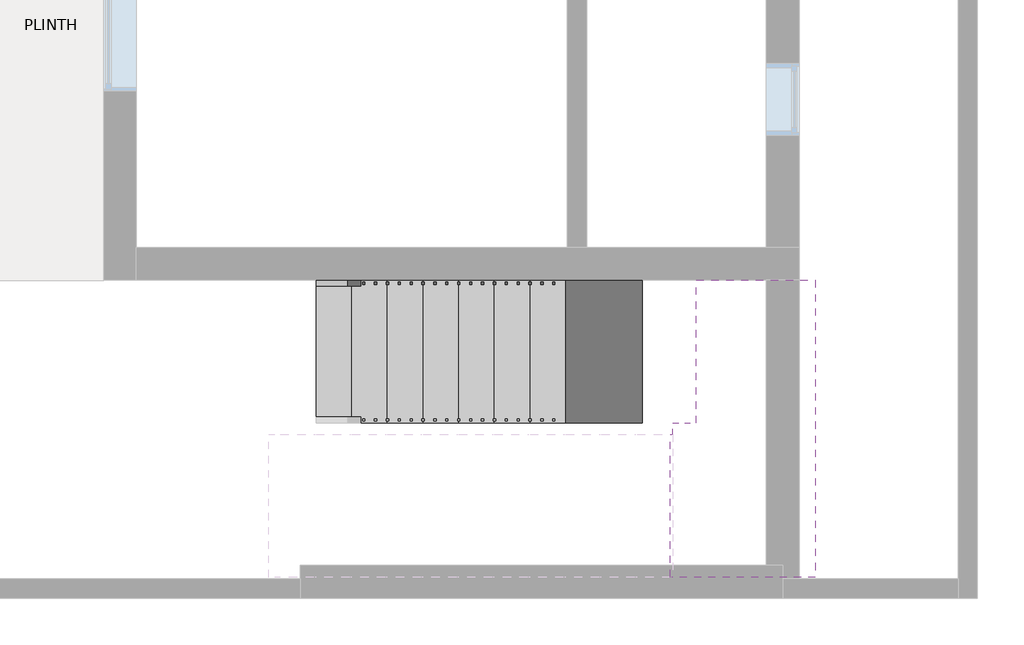
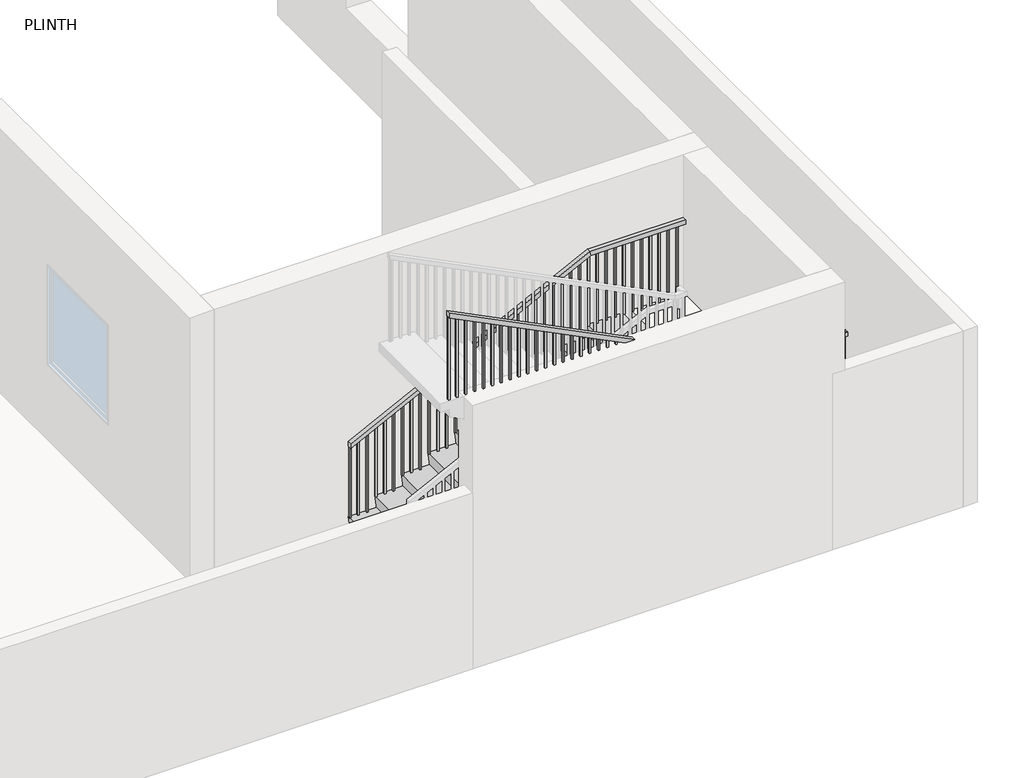
# One storey, part 3 of 3: 1 railing, 1 slab, 1 stair flight.
"""IFC4 building model written with IfcOpenShell, lengths in millimetres."""

from ifc_helpers import new_model, si_unit, frame, origin, place, context, project, spatial, polyline, outline, extrude, faceted_brep, element, save

model = new_model("IFC4")

# Units and contexts
model_context = context("Model", 3, world=origin())
ifc_project = project(units=[si_unit("LENGTHUNIT", "METRE", prefix="MILLI")], contexts=[model_context])

# Site, building, storey
site = spatial("IfcSite", under=ifc_project)
building = spatial("IfcBuilding", under=site)
storey = spatial("IfcBuildingStorey", under=building, Name="PLINTH", Elevation=0.0)

# Railing
placement = place(None, origin())
element("IfcRailing", 1, ObjectType="Handrail - Rectangular", at=placement, inside=storey, context=model_context, shape_type="SolidModel", body=[
    faceted_brep([(-13267.32252, -2786.4806156, 1066.8), (-13267.32252, -2786.4806156, 1010.0038734), (-13267.32252, -2837.2806156, 1010.0038734), (-13267.32252, -2837.2806156, 1066.8), (-10524.12252, -2786.4806156, 2438.4), (-10512.1302667, -2786.4806156, 2387.6), (-10512.1302667, -2837.2806156, 2387.6), (-10524.12252, -2837.2806156, 2438.4), (-9000.12252, -2786.4806156, 2438.4), (-9000.12252, -2786.4806156, 2387.6), (-9050.92252, -2837.2806156, 2387.6), (-9050.92252, -2837.2806156, 2438.4), (-9000.12252, -5326.4806156, 2438.4), (-9000.12252, -5326.4806156, 2387.6), (-9050.92252, -5275.6806156, 2387.6), (-9050.92252, -5275.6806156, 2438.4), (-9914.52252, -5326.4806156, 2438.4), (-9926.5147732, -5326.4806156, 2387.6), (-9926.5147732, -5275.6806156, 2387.6), (-9914.52252, -5275.6806156, 2438.4), (-13572.12252, -5326.4806156, 4267.2), (-13572.12252, -5275.6806156, 4267.2), (-13572.12252, -5275.6806156, 4210.4038734), (-13572.12252, -5326.4806156, 4210.4038734)], [[[0, 1, 2, 3]], [[1, 0, 4, 5]], [[2, 1, 5, 6]], [[3, 2, 6, 7]], [[0, 3, 7, 4]], [[5, 4, 8, 9]], [[6, 5, 9, 10]], [[7, 6, 10, 11]], [[4, 7, 11, 8]], [[9, 8, 12, 13]], [[10, 9, 13, 14]], [[11, 10, 14, 15]], [[8, 11, 15, 12]], [[13, 12, 16, 17]], [[14, 13, 17, 18]], [[15, 14, 18, 19]], [[12, 15, 19, 16]], [[20, 21, 22, 23]], [[17, 16, 20, 23]], [[18, 17, 23, 22]], [[19, 18, 22, 21]], [[16, 19, 21, 20]]]),
    extrude(outline(polyline([(4164.3663734, -13480.04752), (3200.4, -13480.04752), (3200.4, -13460.99752), (4154.8413734, -13460.99752), (4164.3663734, -13480.04752)])), frame((0.0, -5310.6056156, 0.0), z_axis=(0.0, 1.0, 0.0), x_axis=(0.0, 0.0, 1.0)), (0.0, 0.0, 1.0), 19.05),
    extrude(outline(polyline([(4113.5663734, -13378.44752), (3200.4, -13378.44752), (3200.4, -13359.39752), (4104.0413734, -13359.39752), (4113.5663734, -13378.44752)])), frame((0.0, -5310.6056156, 0.0), z_axis=(0.0, 1.0, 0.0), x_axis=(0.0, 0.0, 1.0)), (0.0, 0.0, 1.0), 19.05),
    extrude(outline(polyline([(4062.7663734, -13276.84752), (3200.4, -13276.84752), (3200.4, -13257.79752), (4053.2413734, -13257.79752), (4062.7663734, -13276.84752)])), frame((0.0, -5310.6056156, 0.0), z_axis=(0.0, 1.0, 0.0), x_axis=(0.0, 0.0, 1.0)), (0.0, 0.0, 1.0), 19.05),
    extrude(outline(polyline([(4011.9663734, -13175.24752), (3048.0, -13175.24752), (3048.0, -13156.19752), (4002.4413734, -13156.19752), (4011.9663734, -13175.24752)])), frame((0.0, -5310.6056156, 0.0), z_axis=(0.0, 1.0, 0.0), x_axis=(0.0, 0.0, 1.0)), (0.0, 0.0, 1.0), 19.05),
    extrude(outline(polyline([(3961.1663734, -13073.64752), (3048.0, -13073.64752), (3048.0, -13054.59752), (3951.6413734, -13054.59752), (3961.1663734, -13073.64752)])), frame((0.0, -5310.6056156, 0.0), z_axis=(0.0, 1.0, 0.0), x_axis=(0.0, 0.0, 1.0)), (0.0, 0.0, 1.0), 19.05),
    extrude(outline(polyline([(3910.3663734, -12972.04752), (3048.0, -12972.04752), (3048.0, -12952.99752), (3900.8413734, -12952.99752), (3910.3663734, -12972.04752)])), frame((0.0, -5310.6056156, 0.0), z_axis=(0.0, 1.0, 0.0), x_axis=(0.0, 0.0, 1.0)), (0.0, 0.0, 1.0), 19.05),
    extrude(outline(polyline([(3859.5663734, -12870.44752), (2895.6, -12870.44752), (2895.6, -12851.39752), (3850.0413734, -12851.39752), (3859.5663734, -12870.44752)])), frame((0.0, -5310.6056156, 0.0), z_axis=(0.0, 1.0, 0.0), x_axis=(0.0, 0.0, 1.0)), (0.0, 0.0, 1.0), 19.05),
    extrude(outline(polyline([(3808.7663734, -12768.84752), (2895.6, -12768.84752), (2895.6, -12749.79752), (3799.2413734, -12749.79752), (3808.7663734, -12768.84752)])), frame((0.0, -5310.6056156, 0.0), z_axis=(0.0, 1.0, 0.0), x_axis=(0.0, 0.0, 1.0)), (0.0, 0.0, 1.0), 19.05),
    extrude(outline(polyline([(3757.9663734, -12667.24752), (2895.6, -12667.24752), (2895.6, -12648.19752), (3748.4413734, -12648.19752), (3757.9663734, -12667.24752)])), frame((0.0, -5310.6056156, 0.0), z_axis=(0.0, 1.0, 0.0), x_axis=(0.0, 0.0, 1.0)), (0.0, 0.0, 1.0), 19.05),
    extrude(outline(polyline([(3707.1663734, -12565.64752), (2743.2, -12565.64752), (2743.2, -12546.59752), (3697.6413734, -12546.59752), (3707.1663734, -12565.64752)])), frame((0.0, -5310.6056156, 0.0), z_axis=(0.0, 1.0, 0.0), x_axis=(0.0, 0.0, 1.0)), (0.0, 0.0, 1.0), 19.05),
    extrude(outline(polyline([(3656.3663734, -12464.04752), (2743.2, -12464.04752), (2743.2, -12444.99752), (3646.8413734, -12444.99752), (3656.3663734, -12464.04752)])), frame((0.0, -5310.6056156, 0.0), z_axis=(0.0, 1.0, 0.0), x_axis=(0.0, 0.0, 1.0)), (0.0, 0.0, 1.0), 19.05),
    extrude(outline(polyline([(3605.5663734, -12362.44752), (2743.2, -12362.44752), (2743.2, -12343.39752), (3596.0413734, -12343.39752), (3605.5663734, -12362.44752)])), frame((0.0, -5310.6056156, 0.0), z_axis=(0.0, 1.0, 0.0), x_axis=(0.0, 0.0, 1.0)), (0.0, 0.0, 1.0), 19.05),
    extrude(outline(polyline([(3554.7663734, -12260.84752), (2590.8, -12260.84752), (2590.8, -12241.79752), (3545.2413734, -12241.79752), (3554.7663734, -12260.84752)])), frame((0.0, -5310.6056156, 0.0), z_axis=(0.0, 1.0, 0.0), x_axis=(0.0, 0.0, 1.0)), (0.0, 0.0, 1.0), 19.05),
    extrude(outline(polyline([(3503.9663734, -12159.24752), (2590.8, -12159.24752), (2590.8, -12140.19752), (3494.4413734, -12140.19752), (3503.9663734, -12159.24752)])), frame((0.0, -5310.6056156, 0.0), z_axis=(0.0, 1.0, 0.0), x_axis=(0.0, 0.0, 1.0)), (0.0, 0.0, 1.0), 19.05),
    extrude(outline(polyline([(3453.1663734, -12057.64752), (2590.8, -12057.64752), (2590.8, -12038.59752), (3443.6413734, -12038.59752), (3453.1663734, -12057.64752)])), frame((0.0, -5310.6056156, 0.0), z_axis=(0.0, 1.0, 0.0), x_axis=(0.0, 0.0, 1.0)), (0.0, 0.0, 1.0), 19.05),
    extrude(outline(polyline([(3402.3663734, -11956.04752), (2438.4, -11956.04752), (2438.4, -11936.99752), (3392.8413734, -11936.99752), (3402.3663734, -11956.04752)])), frame((0.0, -5310.6056156, 0.0), z_axis=(0.0, 1.0, 0.0), x_axis=(0.0, 0.0, 1.0)), (0.0, 0.0, 1.0), 19.05),
    extrude(outline(polyline([(3351.5663734, -11854.44752), (2438.4, -11854.44752), (2438.4, -11835.39752), (3342.0413734, -11835.39752), (3351.5663734, -11854.44752)])), frame((0.0, -5310.6056156, 0.0), z_axis=(0.0, 1.0, 0.0), x_axis=(0.0, 0.0, 1.0)), (0.0, 0.0, 1.0), 19.05),
    extrude(outline(polyline([(3300.7663734, -11752.84752), (2438.4, -11752.84752), (2438.4, -11733.79752), (3291.2413734, -11733.79752), (3300.7663734, -11752.84752)])), frame((0.0, -5310.6056156, 0.0), z_axis=(0.0, 1.0, 0.0), x_axis=(0.0, 0.0, 1.0)), (0.0, 0.0, 1.0), 19.05),
    extrude(outline(polyline([(3249.9663734, -11651.24752), (2286.0, -11651.24752), (2286.0, -11632.19752), (3240.4413734, -11632.19752), (3249.9663734, -11651.24752)])), frame((0.0, -5310.6056156, 0.0), z_axis=(0.0, 1.0, 0.0), x_axis=(0.0, 0.0, 1.0)), (0.0, 0.0, 1.0), 19.05),
    extrude(outline(polyline([(3199.1663734, -11549.64752), (2286.0, -11549.64752), (2286.0, -11530.59752), (3189.6413734, -11530.59752), (3199.1663734, -11549.64752)])), frame((0.0, -5310.6056156, 0.0), z_axis=(0.0, 1.0, 0.0), x_axis=(0.0, 0.0, 1.0)), (0.0, 0.0, 1.0), 19.05),
    extrude(outline(polyline([(3148.3663734, -11448.04752), (2286.0, -11448.04752), (2286.0, -11428.99752), (3138.8413734, -11428.99752), (3148.3663734, -11448.04752)])), frame((0.0, -5310.6056156, 0.0), z_axis=(0.0, 1.0, 0.0), x_axis=(0.0, 0.0, 1.0)), (0.0, 0.0, 1.0), 19.05),
    extrude(outline(polyline([(3097.5663734, -11346.44752), (2133.6, -11346.44752), (2133.6, -11327.39752), (3088.0413734, -11327.39752), (3097.5663734, -11346.44752)])), frame((0.0, -5310.6056156, 0.0), z_axis=(0.0, 1.0, 0.0), x_axis=(0.0, 0.0, 1.0)), (0.0, 0.0, 1.0), 19.05),
    extrude(outline(polyline([(3046.7663734, -11244.84752), (2133.6, -11244.84752), (2133.6, -11225.79752), (3037.2413734, -11225.79752), (3046.7663734, -11244.84752)])), frame((0.0, -5310.6056156, 0.0), z_axis=(0.0, 1.0, 0.0), x_axis=(0.0, 0.0, 1.0)), (0.0, 0.0, 1.0), 19.05),
    extrude(outline(polyline([(2995.9663734, -11143.24752), (2133.6, -11143.24752), (2133.6, -11124.19752), (2986.4413734, -11124.19752), (2995.9663734, -11143.24752)])), frame((0.0, -5310.6056156, 0.0), z_axis=(0.0, 1.0, 0.0), x_axis=(0.0, 0.0, 1.0)), (0.0, 0.0, 1.0), 19.05),
    extrude(outline(polyline([(2945.1663734, -11041.64752), (1981.2, -11041.64752), (1981.2, -11022.59752), (2935.6413734, -11022.59752), (2945.1663734, -11041.64752)])), frame((0.0, -5310.6056156, 0.0), z_axis=(0.0, 1.0, 0.0), x_axis=(0.0, 0.0, 1.0)), (0.0, 0.0, 1.0), 19.05),
    extrude(outline(polyline([(2894.3663734, -10940.04752), (1981.2, -10940.04752), (1981.2, -10920.99752), (2884.8413734, -10920.99752), (2894.3663734, -10940.04752)])), frame((0.0, -5310.6056156, 0.0), z_axis=(0.0, 1.0, 0.0), x_axis=(0.0, 0.0, 1.0)), (0.0, 0.0, 1.0), 19.05),
    extrude(outline(polyline([(2843.5663734, -10838.44752), (1981.2, -10838.44752), (1981.2, -10819.39752), (2834.0413734, -10819.39752), (2843.5663734, -10838.44752)])), frame((0.0, -5310.6056156, 0.0), z_axis=(0.0, 1.0, 0.0), x_axis=(0.0, 0.0, 1.0)), (0.0, 0.0, 1.0), 19.05),
    extrude(outline(polyline([(2792.7663734, -10736.84752), (1828.8, -10736.84752), (1828.8, -10717.79752), (2783.2413734, -10717.79752), (2792.7663734, -10736.84752)])), frame((0.0, -5310.6056156, 0.0), z_axis=(0.0, 1.0, 0.0), x_axis=(0.0, 0.0, 1.0)), (0.0, 0.0, 1.0), 19.05),
    extrude(outline(polyline([(2741.9663734, -10635.24752), (1828.8, -10635.24752), (1828.8, -10616.19752), (2732.4413734, -10616.19752), (2741.9663734, -10635.24752)])), frame((0.0, -5310.6056156, 0.0), z_axis=(0.0, 1.0, 0.0), x_axis=(0.0, 0.0, 1.0)), (0.0, 0.0, 1.0), 19.05),
    extrude(outline(polyline([(2691.1663734, -10533.64752), (1828.8, -10533.64752), (1828.8, -10514.59752), (2681.6413734, -10514.59752), (2691.1663734, -10533.64752)])), frame((0.0, -5310.6056156, 0.0), z_axis=(0.0, 1.0, 0.0), x_axis=(0.0, 0.0, 1.0)), (0.0, 0.0, 1.0), 19.05),
    extrude(outline(polyline([(2640.3663734, -10432.04752), (1676.4, -10432.04752), (1676.4, -10412.99752), (2630.8413734, -10412.99752), (2640.3663734, -10432.04752)])), frame((0.0, -5310.6056156, 0.0), z_axis=(0.0, 1.0, 0.0), x_axis=(0.0, 0.0, 1.0)), (0.0, 0.0, 1.0), 19.05),
    extrude(outline(polyline([(2589.5663734, -10330.44752), (1676.4, -10330.44752), (1676.4, -10311.39752), (2580.0413734, -10311.39752), (2589.5663734, -10330.44752)])), frame((0.0, -5310.6056156, 0.0), z_axis=(0.0, 1.0, 0.0), x_axis=(0.0, 0.0, 1.0)), (0.0, 0.0, 1.0), 19.05),
    extrude(outline(polyline([(2538.7663734, -10228.84752), (1676.4, -10228.84752), (1676.4, -10209.79752), (2529.2413734, -10209.79752), (2538.7663734, -10228.84752)])), frame((0.0, -5310.6056156, 0.0), z_axis=(0.0, 1.0, 0.0), x_axis=(0.0, 0.0, 1.0)), (0.0, 0.0, 1.0), 19.05),
    extrude(outline(polyline([(2487.9663734, -10127.24752), (1524.0, -10127.24752), (1524.0, -10108.19752), (2478.4413734, -10108.19752), (2487.9663734, -10127.24752)])), frame((0.0, -5310.6056156, 0.0), z_axis=(0.0, 1.0, 0.0), x_axis=(0.0, 0.0, 1.0)), (0.0, 0.0, 1.0), 19.05),
    extrude(outline(polyline([(2437.1663734, -10025.64752), (1524.0, -10025.64752), (1524.0, -10006.59752), (2427.6413734, -10006.59752), (2437.1663734, -10025.64752)])), frame((0.0, -5310.6056156, 0.0), z_axis=(0.0, 1.0, 0.0), x_axis=(0.0, 0.0, 1.0)), (0.0, 0.0, 1.0), 19.05),
    extrude(outline(polyline([(-9828.79752, -5310.6056156), (-9847.84752, -5310.6056156), (-9847.84752, -5291.5556156), (-9828.79752, -5291.5556156), (-9828.79752, -5310.6056156)])), frame((0.0, 0.0, 1524.0), z_axis=(0.0, 0.0, 1.0), x_axis=(1.0, 0.0, 0.0)), (0.0, 0.0, 1.0), 863.6),
    extrude(outline(polyline([(-9727.19752, -5310.6056156), (-9746.24752, -5310.6056156), (-9746.24752, -5291.5556156), (-9727.19752, -5291.5556156), (-9727.19752, -5310.6056156)])), frame((0.0, 0.0, 1524.0), z_axis=(0.0, 0.0, 1.0), x_axis=(1.0, 0.0, 0.0)), (0.0, 0.0, 1.0), 863.6),
    extrude(outline(polyline([(-9625.59752, -5310.6056156), (-9644.64752, -5310.6056156), (-9644.64752, -5291.5556156), (-9625.59752, -5291.5556156), (-9625.59752, -5310.6056156)])), frame((0.0, 0.0, 1524.0), z_axis=(0.0, 0.0, 1.0), x_axis=(1.0, 0.0, 0.0)), (0.0, 0.0, 1.0), 863.6),
    extrude(outline(polyline([(-9523.99752, -5310.6056156), (-9543.04752, -5310.6056156), (-9543.04752, -5291.5556156), (-9523.99752, -5291.5556156), (-9523.99752, -5310.6056156)])), frame((0.0, 0.0, 1524.0), z_axis=(0.0, 0.0, 1.0), x_axis=(1.0, 0.0, 0.0)), (0.0, 0.0, 1.0), 863.6),
    extrude(outline(polyline([(-9422.39752, -5310.6056156), (-9441.44752, -5310.6056156), (-9441.44752, -5291.5556156), (-9422.39752, -5291.5556156), (-9422.39752, -5310.6056156)])), frame((0.0, 0.0, 1524.0), z_axis=(0.0, 0.0, 1.0), x_axis=(1.0, 0.0, 0.0)), (0.0, 0.0, 1.0), 863.6),
    extrude(outline(polyline([(-9320.79752, -5310.6056156), (-9339.84752, -5310.6056156), (-9339.84752, -5291.5556156), (-9320.79752, -5291.5556156), (-9320.79752, -5310.6056156)])), frame((0.0, 0.0, 1524.0), z_axis=(0.0, 0.0, 1.0), x_axis=(1.0, 0.0, 0.0)), (0.0, 0.0, 1.0), 863.6),
    extrude(outline(polyline([(-9219.19752, -5310.6056156), (-9238.24752, -5310.6056156), (-9238.24752, -5291.5556156), (-9219.19752, -5291.5556156), (-9219.19752, -5310.6056156)])), frame((0.0, 0.0, 1524.0), z_axis=(0.0, 0.0, 1.0), x_axis=(1.0, 0.0, 0.0)), (0.0, 0.0, 1.0), 863.6),
    extrude(outline(polyline([(-9117.59752, -5310.6056156), (-9136.64752, -5310.6056156), (-9136.64752, -5291.5556156), (-9117.59752, -5291.5556156), (-9117.59752, -5310.6056156)])), frame((0.0, 0.0, 1524.0), z_axis=(0.0, 0.0, 1.0), x_axis=(1.0, 0.0, 0.0)), (0.0, 0.0, 1.0), 863.6),
    extrude(outline(polyline([(-9015.99752, -5240.7556156), (-9015.99752, -5259.8056156), (-9035.04752, -5259.8056156), (-9035.04752, -5240.7556156), (-9015.99752, -5240.7556156)])), frame((0.0, 0.0, 1524.0), z_axis=(0.0, 0.0, 1.0), x_axis=(1.0, 0.0, 0.0)), (0.0, 0.0, 1.0), 863.6),
    extrude(outline(polyline([(-9015.99752, -5139.1556156), (-9015.99752, -5158.2056156), (-9035.04752, -5158.2056156), (-9035.04752, -5139.1556156), (-9015.99752, -5139.1556156)])), frame((0.0, 0.0, 1524.0), z_axis=(0.0, 0.0, 1.0), x_axis=(1.0, 0.0, 0.0)), (0.0, 0.0, 1.0), 863.6),
    extrude(outline(polyline([(-9015.99752, -5037.5556156), (-9015.99752, -5056.6056156), (-9035.04752, -5056.6056156), (-9035.04752, -5037.5556156), (-9015.99752, -5037.5556156)])), frame((0.0, 0.0, 1524.0), z_axis=(0.0, 0.0, 1.0), x_axis=(1.0, 0.0, 0.0)), (0.0, 0.0, 1.0), 863.6),
    extrude(outline(polyline([(-9015.99752, -4935.9556156), (-9015.99752, -4955.0056156), (-9035.04752, -4955.0056156), (-9035.04752, -4935.9556156), (-9015.99752, -4935.9556156)])), frame((0.0, 0.0, 1524.0), z_axis=(0.0, 0.0, 1.0), x_axis=(1.0, 0.0, 0.0)), (0.0, 0.0, 1.0), 863.6),
    extrude(outline(polyline([(-9015.99752, -4834.3556156), (-9015.99752, -4853.4056156), (-9035.04752, -4853.4056156), (-9035.04752, -4834.3556156), (-9015.99752, -4834.3556156)])), frame((0.0, 0.0, 1524.0), z_axis=(0.0, 0.0, 1.0), x_axis=(1.0, 0.0, 0.0)), (0.0, 0.0, 1.0), 863.6),
    extrude(outline(polyline([(-9015.99752, -4732.7556156), (-9015.99752, -4751.8056156), (-9035.04752, -4751.8056156), (-9035.04752, -4732.7556156), (-9015.99752, -4732.7556156)])), frame((0.0, 0.0, 1524.0), z_axis=(0.0, 0.0, 1.0), x_axis=(1.0, 0.0, 0.0)), (0.0, 0.0, 1.0), 863.6),
    extrude(outline(polyline([(-9015.99752, -4631.1556156), (-9015.99752, -4650.2056156), (-9035.04752, -4650.2056156), (-9035.04752, -4631.1556156), (-9015.99752, -4631.1556156)])), frame((0.0, 0.0, 1524.0), z_axis=(0.0, 0.0, 1.0), x_axis=(1.0, 0.0, 0.0)), (0.0, 0.0, 1.0), 863.6),
    extrude(outline(polyline([(-9015.99752, -4529.5556156), (-9015.99752, -4548.6056156), (-9035.04752, -4548.6056156), (-9035.04752, -4529.5556156), (-9015.99752, -4529.5556156)])), frame((0.0, 0.0, 1524.0), z_axis=(0.0, 0.0, 1.0), x_axis=(1.0, 0.0, 0.0)), (0.0, 0.0, 1.0), 863.6),
    extrude(outline(polyline([(-9015.99752, -4427.9556156), (-9015.99752, -4447.0056156), (-9035.04752, -4447.0056156), (-9035.04752, -4427.9556156), (-9015.99752, -4427.9556156)])), frame((0.0, 0.0, 1524.0), z_axis=(0.0, 0.0, 1.0), x_axis=(1.0, 0.0, 0.0)), (0.0, 0.0, 1.0), 863.6),
    extrude(outline(polyline([(-9015.99752, -4326.3556156), (-9015.99752, -4345.4056156), (-9035.04752, -4345.4056156), (-9035.04752, -4326.3556156), (-9015.99752, -4326.3556156)])), frame((0.0, 0.0, 1524.0), z_axis=(0.0, 0.0, 1.0), x_axis=(1.0, 0.0, 0.0)), (0.0, 0.0, 1.0), 863.6),
    extrude(outline(polyline([(-9015.99752, -4224.7556156), (-9015.99752, -4243.8056156), (-9035.04752, -4243.8056156), (-9035.04752, -4224.7556156), (-9015.99752, -4224.7556156)])), frame((0.0, 0.0, 1524.0), z_axis=(0.0, 0.0, 1.0), x_axis=(1.0, 0.0, 0.0)), (0.0, 0.0, 1.0), 863.6),
    extrude(outline(polyline([(-9015.99752, -4123.1556156), (-9015.99752, -4142.2056156), (-9035.04752, -4142.2056156), (-9035.04752, -4123.1556156), (-9015.99752, -4123.1556156)])), frame((0.0, 0.0, 1524.0), z_axis=(0.0, 0.0, 1.0), x_axis=(1.0, 0.0, 0.0)), (0.0, 0.0, 1.0), 863.6),
    extrude(outline(polyline([(-9015.99752, -4021.5556156), (-9015.99752, -4040.6056156), (-9035.04752, -4040.6056156), (-9035.04752, -4021.5556156), (-9015.99752, -4021.5556156)])), frame((0.0, 0.0, 1524.0), z_axis=(0.0, 0.0, 1.0), x_axis=(1.0, 0.0, 0.0)), (0.0, 0.0, 1.0), 863.6),
    extrude(outline(polyline([(-9015.99752, -3919.9556156), (-9015.99752, -3939.0056156), (-9035.04752, -3939.0056156), (-9035.04752, -3919.9556156), (-9015.99752, -3919.9556156)])), frame((0.0, 0.0, 1524.0), z_axis=(0.0, 0.0, 1.0), x_axis=(1.0, 0.0, 0.0)), (0.0, 0.0, 1.0), 863.6),
    extrude(outline(polyline([(-9015.99752, -3818.3556156), (-9015.99752, -3837.4056156), (-9035.04752, -3837.4056156), (-9035.04752, -3818.3556156), (-9015.99752, -3818.3556156)])), frame((0.0, 0.0, 1524.0), z_axis=(0.0, 0.0, 1.0), x_axis=(1.0, 0.0, 0.0)), (0.0, 0.0, 1.0), 863.6),
    extrude(outline(polyline([(-9015.99752, -3716.7556156), (-9015.99752, -3735.8056156), (-9035.04752, -3735.8056156), (-9035.04752, -3716.7556156), (-9015.99752, -3716.7556156)])), frame((0.0, 0.0, 1524.0), z_axis=(0.0, 0.0, 1.0), x_axis=(1.0, 0.0, 0.0)), (0.0, 0.0, 1.0), 863.6),
    extrude(outline(polyline([(-9015.99752, -3615.1556156), (-9015.99752, -3634.2056156), (-9035.04752, -3634.2056156), (-9035.04752, -3615.1556156), (-9015.99752, -3615.1556156)])), frame((0.0, 0.0, 1524.0), z_axis=(0.0, 0.0, 1.0), x_axis=(1.0, 0.0, 0.0)), (0.0, 0.0, 1.0), 863.6),
    extrude(outline(polyline([(-9015.99752, -3513.5556156), (-9015.99752, -3532.6056156), (-9035.04752, -3532.6056156), (-9035.04752, -3513.5556156), (-9015.99752, -3513.5556156)])), frame((0.0, 0.0, 1524.0), z_axis=(0.0, 0.0, 1.0), x_axis=(1.0, 0.0, 0.0)), (0.0, 0.0, 1.0), 863.6),
    extrude(outline(polyline([(-9015.99752, -3411.9556156), (-9015.99752, -3431.0056156), (-9035.04752, -3431.0056156), (-9035.04752, -3411.9556156), (-9015.99752, -3411.9556156)])), frame((0.0, 0.0, 1524.0), z_axis=(0.0, 0.0, 1.0), x_axis=(1.0, 0.0, 0.0)), (0.0, 0.0, 1.0), 863.6),
    extrude(outline(polyline([(-9015.99752, -3310.3556156), (-9015.99752, -3329.4056156), (-9035.04752, -3329.4056156), (-9035.04752, -3310.3556156), (-9015.99752, -3310.3556156)])), frame((0.0, 0.0, 1524.0), z_axis=(0.0, 0.0, 1.0), x_axis=(1.0, 0.0, 0.0)), (0.0, 0.0, 1.0), 863.6),
    extrude(outline(polyline([(-9015.99752, -3208.7556156), (-9015.99752, -3227.8056156), (-9035.04752, -3227.8056156), (-9035.04752, -3208.7556156), (-9015.99752, -3208.7556156)])), frame((0.0, 0.0, 1524.0), z_axis=(0.0, 0.0, 1.0), x_axis=(1.0, 0.0, 0.0)), (0.0, 0.0, 1.0), 863.6),
    extrude(outline(polyline([(-9015.99752, -3107.1556156), (-9015.99752, -3126.2056156), (-9035.04752, -3126.2056156), (-9035.04752, -3107.1556156), (-9015.99752, -3107.1556156)])), frame((0.0, 0.0, 1524.0), z_axis=(0.0, 0.0, 1.0), x_axis=(1.0, 0.0, 0.0)), (0.0, 0.0, 1.0), 863.6),
    extrude(outline(polyline([(-9015.99752, -3005.5556156), (-9015.99752, -3024.6056156), (-9035.04752, -3024.6056156), (-9035.04752, -3005.5556156), (-9015.99752, -3005.5556156)])), frame((0.0, 0.0, 1524.0), z_axis=(0.0, 0.0, 1.0), x_axis=(1.0, 0.0, 0.0)), (0.0, 0.0, 1.0), 863.6),
    extrude(outline(polyline([(-9015.99752, -2903.9556156), (-9015.99752, -2923.0056156), (-9035.04752, -2923.0056156), (-9035.04752, -2903.9556156), (-9015.99752, -2903.9556156)])), frame((0.0, 0.0, 1524.0), z_axis=(0.0, 0.0, 1.0), x_axis=(1.0, 0.0, 0.0)), (0.0, 0.0, 1.0), 863.6),
    extrude(outline(polyline([(-9111.24752, -2802.3556156), (-9092.19752, -2802.3556156), (-9092.19752, -2821.4056156), (-9111.24752, -2821.4056156), (-9111.24752, -2802.3556156)])), frame((0.0, 0.0, 1524.0), z_axis=(0.0, 0.0, 1.0), x_axis=(1.0, 0.0, 0.0)), (0.0, 0.0, 1.0), 863.6),
    extrude(outline(polyline([(-9212.84752, -2802.3556156), (-9193.79752, -2802.3556156), (-9193.79752, -2821.4056156), (-9212.84752, -2821.4056156), (-9212.84752, -2802.3556156)])), frame((0.0, 0.0, 1524.0), z_axis=(0.0, 0.0, 1.0), x_axis=(1.0, 0.0, 0.0)), (0.0, 0.0, 1.0), 863.6),
    extrude(outline(polyline([(-9314.44752, -2802.3556156), (-9295.39752, -2802.3556156), (-9295.39752, -2821.4056156), (-9314.44752, -2821.4056156), (-9314.44752, -2802.3556156)])), frame((0.0, 0.0, 1524.0), z_axis=(0.0, 0.0, 1.0), x_axis=(1.0, 0.0, 0.0)), (0.0, 0.0, 1.0), 863.6),
    extrude(outline(polyline([(-9416.04752, -2802.3556156), (-9396.99752, -2802.3556156), (-9396.99752, -2821.4056156), (-9416.04752, -2821.4056156), (-9416.04752, -2802.3556156)])), frame((0.0, 0.0, 1524.0), z_axis=(0.0, 0.0, 1.0), x_axis=(1.0, 0.0, 0.0)), (0.0, 0.0, 1.0), 863.6),
    extrude(outline(polyline([(-9517.64752, -2802.3556156), (-9498.59752, -2802.3556156), (-9498.59752, -2821.4056156), (-9517.64752, -2821.4056156), (-9517.64752, -2802.3556156)])), frame((0.0, 0.0, 1524.0), z_axis=(0.0, 0.0, 1.0), x_axis=(1.0, 0.0, 0.0)), (0.0, 0.0, 1.0), 863.6),
    extrude(outline(polyline([(-9619.24752, -2802.3556156), (-9600.19752, -2802.3556156), (-9600.19752, -2821.4056156), (-9619.24752, -2821.4056156), (-9619.24752, -2802.3556156)])), frame((0.0, 0.0, 1524.0), z_axis=(0.0, 0.0, 1.0), x_axis=(1.0, 0.0, 0.0)), (0.0, 0.0, 1.0), 863.6),
    extrude(outline(polyline([(-9720.84752, -2802.3556156), (-9701.79752, -2802.3556156), (-9701.79752, -2821.4056156), (-9720.84752, -2821.4056156), (-9720.84752, -2802.3556156)])), frame((0.0, 0.0, 1524.0), z_axis=(0.0, 0.0, 1.0), x_axis=(1.0, 0.0, 0.0)), (0.0, 0.0, 1.0), 863.6),
    extrude(outline(polyline([(-9822.44752, -2802.3556156), (-9803.39752, -2802.3556156), (-9803.39752, -2821.4056156), (-9822.44752, -2821.4056156), (-9822.44752, -2802.3556156)])), frame((0.0, 0.0, 1524.0), z_axis=(0.0, 0.0, 1.0), x_axis=(1.0, 0.0, 0.0)), (0.0, 0.0, 1.0), 863.6),
    extrude(outline(polyline([(-9924.04752, -2802.3556156), (-9904.99752, -2802.3556156), (-9904.99752, -2821.4056156), (-9924.04752, -2821.4056156), (-9924.04752, -2802.3556156)])), frame((0.0, 0.0, 1524.0), z_axis=(0.0, 0.0, 1.0), x_axis=(1.0, 0.0, 0.0)), (0.0, 0.0, 1.0), 863.6),
    extrude(outline(polyline([(-10025.64752, -2802.3556156), (-10006.59752, -2802.3556156), (-10006.59752, -2821.4056156), (-10025.64752, -2821.4056156), (-10025.64752, -2802.3556156)])), frame((0.0, 0.0, 1524.0), z_axis=(0.0, 0.0, 1.0), x_axis=(1.0, 0.0, 0.0)), (0.0, 0.0, 1.0), 863.6),
    extrude(outline(polyline([(-10127.24752, -2802.3556156), (-10108.19752, -2802.3556156), (-10108.19752, -2821.4056156), (-10127.24752, -2821.4056156), (-10127.24752, -2802.3556156)])), frame((0.0, 0.0, 1524.0), z_axis=(0.0, 0.0, 1.0), x_axis=(1.0, 0.0, 0.0)), (0.0, 0.0, 1.0), 863.6),
    extrude(outline(polyline([(-10228.84752, -2802.3556156), (-10209.79752, -2802.3556156), (-10209.79752, -2821.4056156), (-10228.84752, -2821.4056156), (-10228.84752, -2802.3556156)])), frame((0.0, 0.0, 1524.0), z_axis=(0.0, 0.0, 1.0), x_axis=(1.0, 0.0, 0.0)), (0.0, 0.0, 1.0), 863.6),
    extrude(outline(polyline([(-10330.44752, -2802.3556156), (-10311.39752, -2802.3556156), (-10311.39752, -2821.4056156), (-10330.44752, -2821.4056156), (-10330.44752, -2802.3556156)])), frame((0.0, 0.0, 1524.0), z_axis=(0.0, 0.0, 1.0), x_axis=(1.0, 0.0, 0.0)), (0.0, 0.0, 1.0), 863.6),
    extrude(outline(polyline([(-10432.04752, -2802.3556156), (-10412.99752, -2802.3556156), (-10412.99752, -2821.4056156), (-10432.04752, -2821.4056156), (-10432.04752, -2802.3556156)])), frame((0.0, 0.0, 1524.0), z_axis=(0.0, 0.0, 1.0), x_axis=(1.0, 0.0, 0.0)), (0.0, 0.0, 1.0), 863.6),
    extrude(outline(polyline([(2326.0413734, -10635.24752), (1371.6, -10635.24752), (1371.6, -10616.19752), (2335.5663734, -10616.19752), (2326.0413734, -10635.24752)])), frame((0.0, -2821.4056156, 0.0), z_axis=(0.0, 1.0, 0.0), x_axis=(0.0, 0.0, 1.0)), (0.0, 0.0, 1.0), 19.05),
    extrude(outline(polyline([(2275.2413734, -10736.84752), (1371.6, -10736.84752), (1371.6, -10717.79752), (2284.7663734, -10717.79752), (2275.2413734, -10736.84752)])), frame((0.0, -2821.4056156, 0.0), z_axis=(0.0, 1.0, 0.0), x_axis=(0.0, 0.0, 1.0)), (0.0, 0.0, 1.0), 19.05),
    extrude(outline(polyline([(2224.4413734, -10838.44752), (1371.6, -10838.44752), (1371.6, -10819.39752), (2233.9663734, -10819.39752), (2224.4413734, -10838.44752)])), frame((0.0, -2821.4056156, 0.0), z_axis=(0.0, 1.0, 0.0), x_axis=(0.0, 0.0, 1.0)), (0.0, 0.0, 1.0), 19.05),
    extrude(outline(polyline([(2173.6413734, -10940.04752), (1219.2, -10940.04752), (1219.2, -10920.99752), (2183.1663734, -10920.99752), (2173.6413734, -10940.04752)])), frame((0.0, -2821.4056156, 0.0), z_axis=(0.0, 1.0, 0.0), x_axis=(0.0, 0.0, 1.0)), (0.0, 0.0, 1.0), 19.05),
    extrude(outline(polyline([(2122.8413734, -11041.64752), (1219.2, -11041.64752), (1219.2, -11022.59752), (2132.3663734, -11022.59752), (2122.8413734, -11041.64752)])), frame((0.0, -2821.4056156, 0.0), z_axis=(0.0, 1.0, 0.0), x_axis=(0.0, 0.0, 1.0)), (0.0, 0.0, 1.0), 19.05),
    extrude(outline(polyline([(2072.0413734, -11143.24752), (1219.2, -11143.24752), (1219.2, -11124.19752), (2081.5663734, -11124.19752), (2072.0413734, -11143.24752)])), frame((0.0, -2821.4056156, 0.0), z_axis=(0.0, 1.0, 0.0), x_axis=(0.0, 0.0, 1.0)), (0.0, 0.0, 1.0), 19.05),
    extrude(outline(polyline([(2021.2413734, -11244.84752), (1066.8, -11244.84752), (1066.8, -11225.79752), (2030.7663734, -11225.79752), (2021.2413734, -11244.84752)])), frame((0.0, -2821.4056156, 0.0), z_axis=(0.0, 1.0, 0.0), x_axis=(0.0, 0.0, 1.0)), (0.0, 0.0, 1.0), 19.05),
    extrude(outline(polyline([(1970.4413734, -11346.44752), (1066.8, -11346.44752), (1066.8, -11327.39752), (1979.9663734, -11327.39752), (1970.4413734, -11346.44752)])), frame((0.0, -2821.4056156, 0.0), z_axis=(0.0, 1.0, 0.0), x_axis=(0.0, 0.0, 1.0)), (0.0, 0.0, 1.0), 19.05),
    extrude(outline(polyline([(1919.6413734, -11448.04752), (1066.8, -11448.04752), (1066.8, -11428.99752), (1929.1663734, -11428.99752), (1919.6413734, -11448.04752)])), frame((0.0, -2821.4056156, 0.0), z_axis=(0.0, 1.0, 0.0), x_axis=(0.0, 0.0, 1.0)), (0.0, 0.0, 1.0), 19.05),
    extrude(outline(polyline([(1868.8413734, -11549.64752), (914.4, -11549.64752), (914.4, -11530.59752), (1878.3663734, -11530.59752), (1868.8413734, -11549.64752)])), frame((0.0, -2821.4056156, 0.0), z_axis=(0.0, 1.0, 0.0), x_axis=(0.0, 0.0, 1.0)), (0.0, 0.0, 1.0), 19.05),
    extrude(outline(polyline([(1818.0413734, -11651.24752), (914.4, -11651.24752), (914.4, -11632.19752), (1827.5663734, -11632.19752), (1818.0413734, -11651.24752)])), frame((0.0, -2821.4056156, 0.0), z_axis=(0.0, 1.0, 0.0), x_axis=(0.0, 0.0, 1.0)), (0.0, 0.0, 1.0), 19.05),
    extrude(outline(polyline([(1767.2413734, -11752.84752), (914.4, -11752.84752), (914.4, -11733.79752), (1776.7663734, -11733.79752), (1767.2413734, -11752.84752)])), frame((0.0, -2821.4056156, 0.0), z_axis=(0.0, 1.0, 0.0), x_axis=(0.0, 0.0, 1.0)), (0.0, 0.0, 1.0), 19.05),
    extrude(outline(polyline([(1716.4413734, -11854.44752), (762.0, -11854.44752), (762.0, -11835.39752), (1725.9663734, -11835.39752), (1716.4413734, -11854.44752)])), frame((0.0, -2821.4056156, 0.0), z_axis=(0.0, 1.0, 0.0), x_axis=(0.0, 0.0, 1.0)), (0.0, 0.0, 1.0), 19.05),
    extrude(outline(polyline([(1665.6413734, -11956.04752), (762.0, -11956.04752), (762.0, -11936.99752), (1675.1663734, -11936.99752), (1665.6413734, -11956.04752)])), frame((0.0, -2821.4056156, 0.0), z_axis=(0.0, 1.0, 0.0), x_axis=(0.0, 0.0, 1.0)), (0.0, 0.0, 1.0), 19.05),
    extrude(outline(polyline([(1614.8413734, -12057.64752), (762.0, -12057.64752), (762.0, -12038.59752), (1624.3663734, -12038.59752), (1614.8413734, -12057.64752)])), frame((0.0, -2821.4056156, 0.0), z_axis=(0.0, 1.0, 0.0), x_axis=(0.0, 0.0, 1.0)), (0.0, 0.0, 1.0), 19.05),
    extrude(outline(polyline([(1564.0413734, -12159.24752), (609.6, -12159.24752), (609.6, -12140.19752), (1573.5663734, -12140.19752), (1564.0413734, -12159.24752)])), frame((0.0, -2821.4056156, 0.0), z_axis=(0.0, 1.0, 0.0), x_axis=(0.0, 0.0, 1.0)), (0.0, 0.0, 1.0), 19.05),
    extrude(outline(polyline([(1513.2413734, -12260.84752), (609.6, -12260.84752), (609.6, -12241.79752), (1522.7663734, -12241.79752), (1513.2413734, -12260.84752)])), frame((0.0, -2821.4056156, 0.0), z_axis=(0.0, 1.0, 0.0), x_axis=(0.0, 0.0, 1.0)), (0.0, 0.0, 1.0), 19.05),
    extrude(outline(polyline([(1462.4413734, -12362.44752), (609.6, -12362.44752), (609.6, -12343.39752), (1471.9663734, -12343.39752), (1462.4413734, -12362.44752)])), frame((0.0, -2821.4056156, 0.0), z_axis=(0.0, 1.0, 0.0), x_axis=(0.0, 0.0, 1.0)), (0.0, 0.0, 1.0), 19.05),
    extrude(outline(polyline([(1411.6413734, -12464.04752), (457.2, -12464.04752), (457.2, -12444.99752), (1421.1663734, -12444.99752), (1411.6413734, -12464.04752)])), frame((0.0, -2821.4056156, 0.0), z_axis=(0.0, 1.0, 0.0), x_axis=(0.0, 0.0, 1.0)), (0.0, 0.0, 1.0), 19.05),
    extrude(outline(polyline([(1360.8413734, -12565.64752), (457.2, -12565.64752), (457.2, -12546.59752), (1370.3663734, -12546.59752), (1360.8413734, -12565.64752)])), frame((0.0, -2821.4056156, 0.0), z_axis=(0.0, 1.0, 0.0), x_axis=(0.0, 0.0, 1.0)), (0.0, 0.0, 1.0), 19.05),
    extrude(outline(polyline([(1310.0413734, -12667.24752), (457.2, -12667.24752), (457.2, -12648.19752), (1319.5663734, -12648.19752), (1310.0413734, -12667.24752)])), frame((0.0, -2821.4056156, 0.0), z_axis=(0.0, 1.0, 0.0), x_axis=(0.0, 0.0, 1.0)), (0.0, 0.0, 1.0), 19.05),
    extrude(outline(polyline([(1259.2413734, -12768.84752), (304.8, -12768.84752), (304.8, -12749.79752), (1268.7663734, -12749.79752), (1259.2413734, -12768.84752)])), frame((0.0, -2821.4056156, 0.0), z_axis=(0.0, 1.0, 0.0), x_axis=(0.0, 0.0, 1.0)), (0.0, 0.0, 1.0), 19.05),
    extrude(outline(polyline([(1208.4413734, -12870.44752), (304.8, -12870.44752), (304.8, -12851.39752), (1217.9663734, -12851.39752), (1208.4413734, -12870.44752)])), frame((0.0, -2821.4056156, 0.0), z_axis=(0.0, 1.0, 0.0), x_axis=(0.0, 0.0, 1.0)), (0.0, 0.0, 1.0), 19.05),
    extrude(outline(polyline([(1157.6413734, -12972.04752), (304.8, -12972.04752), (304.8, -12952.99752), (1167.1663734, -12952.99752), (1157.6413734, -12972.04752)])), frame((0.0, -2821.4056156, 0.0), z_axis=(0.0, 1.0, 0.0), x_axis=(0.0, 0.0, 1.0)), (0.0, 0.0, 1.0), 19.05),
    extrude(outline(polyline([(1106.8413734, -13073.64752), (152.4, -13073.64752), (152.4, -13054.59752), (1116.3663734, -13054.59752), (1106.8413734, -13073.64752)])), frame((0.0, -2821.4056156, 0.0), z_axis=(0.0, 1.0, 0.0), x_axis=(0.0, 0.0, 1.0)), (0.0, 0.0, 1.0), 19.05),
    extrude(outline(polyline([(1056.0413734, -13175.24752), (152.4, -13175.24752), (152.4, -13156.19752), (1065.5663734, -13156.19752), (1056.0413734, -13175.24752)])), frame((0.0, -2821.4056156, 0.0), z_axis=(0.0, 1.0, 0.0), x_axis=(0.0, 0.0, 1.0)), (0.0, 0.0, 1.0), 19.05),
    extrude(outline(polyline([(-9904.99752, -5310.6056156), (-9924.04752, -5310.6056156), (-9924.04752, -5291.5556156), (-9904.99752, -5291.5556156), (-9904.99752, -5310.6056156)])), frame((0.0, 0.0, 1524.0), z_axis=(0.0, 0.0, 1.0), x_axis=(1.0, 0.0, 0.0)), (0.0, 0.0, 1.0), 863.6),
    extrude(outline(polyline([(-9015.99752, -5291.5556156), (-9015.99752, -5310.6056156), (-9035.04752, -5310.6056156), (-9035.04752, -5291.5556156), (-9015.99752, -5291.5556156)])), frame((0.0, 0.0, 1524.0), z_axis=(0.0, 0.0, 1.0), x_axis=(1.0, 0.0, 0.0)), (0.0, 0.0, 1.0), 863.6),
    extrude(outline(polyline([(-9035.04752, -2802.3556156), (-9015.99752, -2802.3556156), (-9015.99752, -2821.4056156), (-9035.04752, -2821.4056156), (-9035.04752, -2802.3556156)])), frame((0.0, 0.0, 1524.0), z_axis=(0.0, 0.0, 1.0), x_axis=(1.0, 0.0, 0.0)), (0.0, 0.0, 1.0), 863.6),
    extrude(outline(polyline([(2376.8413734, -10533.64752), (1524.0, -10533.64752), (1524.0, -10514.59752), (2386.3663734, -10514.59752), (2376.8413734, -10533.64752)])), frame((0.0, -2821.4056156, 0.0), z_axis=(0.0, 1.0, 0.0), x_axis=(0.0, 0.0, 1.0)), (0.0, 0.0, 1.0), 19.05),
    extrude(outline(polyline([(4210.4038734, -13572.12252), (3200.4, -13572.12252), (3200.4, -13553.07252), (4200.8788734, -13553.07252), (4210.4038734, -13572.12252)])), frame((0.0, -5310.6056156, 0.0), z_axis=(0.0, 1.0, 0.0), x_axis=(0.0, 0.0, 1.0)), (0.0, 0.0, 1.0), 19.05),
    extrude(outline(polyline([(1010.0038734, -13267.32252), (152.4, -13267.32252), (152.4, -13248.27252), (1019.5288734, -13248.27252), (1010.0038734, -13267.32252)])), frame((0.0, -2821.4056156, 0.0), z_axis=(0.0, 1.0, 0.0), x_axis=(0.0, 0.0, 1.0)), (0.0, 0.0, 1.0), 19.05),
])

# Slab
element("IfcSlab", 2, ObjectType="8\" Thickness", at=placement, inside=storey, context=model_context, shape_type="Brep", body=[
    faceted_brep([(-10219.32252, -4107.2806156, 1524.0), (-10238.37252, -4107.2806156, 1524.0), (-10238.37252, -5326.4806156, 1524.0), (-10219.32252, -5326.4806156, 1524.0), (-9000.12252, -5326.4806156, 1524.0), (-9000.12252, -2786.4806156, 1524.0), (-10016.12252, -2786.4806156, 1524.0), (-10016.12252, -4007.2681156, 1524.0), (-10219.32252, -4007.2681156, 1524.0), (-10219.32252, -4107.2806156, 1320.8), (-10219.32252, -4007.2681156, 1320.8), (-10238.37252, -4107.2806156, 1320.8), (-10238.37252, -5326.4806156, 1320.8), (-10219.32252, -5326.4806156, 1320.8), (-9000.12252, -5326.4806156, 1320.8), (-9000.12252, -2786.4806156, 1320.8), (-10016.12252, -2786.4806156, 1320.8), (-10117.72252, -4007.2681156, 1320.8), (-10016.12252, -4007.2681156, 1320.8)], [[[0, 1, 2, 3, 4, 5, 6, 7, 8]], [[9, 0, 8, 10]], [[1, 0, 9, 11]], [[2, 1, 11, 12]], [[3, 2, 12, 13]], [[4, 3, 13, 14]], [[5, 4, 14, 15]], [[5, 15, 16, 6]], [[11, 9, 10, 17, 18, 16, 15, 14, 13, 12]], [[7, 18, 17, 10, 8]], [[18, 7, 6, 16]]]),
])

# Stair flight
element("IfcStairFlight", 3, ObjectType="3/4\" Nosing 6 1/2\" Depth", at=placement, inside=storey, context=model_context, shape_type="Brep", body=[
    faceted_brep([(-13267.32252, -4005.6806156, 152.4), (-13267.32252, -2786.4806156, 152.4), (-13248.27252, -2786.4806156, 0.0), (-13248.27252, -4005.6806156, 0.0), (-12943.47252, -4005.6806156, 152.4), (-12943.47252, -2786.4806156, 152.4), (-12943.47252, -2786.4806156, 0.0), (-12943.47252, -4005.6806156, 0.0), (-12962.52252, -2786.4806156, 304.8), (-12962.52252, -4005.6806156, 304.8), (-12638.67252, -4005.6806156, 304.8), (-12638.67252, -2786.4806156, 304.8), (-12638.67252, -2786.4806156, 120.2125885), (-12879.0976969, -2786.4806156, 0.0), (-12879.0976969, -4005.6806156, 0.0), (-12638.67252, -4005.6806156, 120.2125885), (-12657.72252, -2786.4806156, 457.2), (-12657.72252, -4005.6806156, 457.2), (-12333.87252, -4005.6806156, 457.2), (-12333.87252, -2786.4806156, 457.2), (-12333.87252, -2786.4806156, 272.6125885), (-12333.87252, -4005.6806156, 272.6125885), (-12352.92252, -2786.4806156, 609.6), (-12352.92252, -4005.6806156, 609.6), (-12029.07252, -4005.6806156, 609.6), (-12029.07252, -2786.4806156, 609.6), (-12029.07252, -2786.4806156, 425.0125885), (-12029.07252, -4005.6806156, 425.0125885), (-12048.12252, -2786.4806156, 762.0), (-12048.12252, -4005.6806156, 762.0), (-11724.27252, -4005.6806156, 762.0), (-11724.27252, -2786.4806156, 762.0), (-11724.27252, -2786.4806156, 577.4125885), (-11724.27252, -4005.6806156, 577.4125885), (-11743.32252, -2786.4806156, 914.4), (-11743.32252, -4005.6806156, 914.4), (-11419.47252, -4005.6806156, 914.4), (-11419.47252, -2786.4806156, 914.4), (-11419.47252, -2786.4806156, 729.8125885), (-11419.47252, -4005.6806156, 729.8125885), (-11438.52252, -2786.4806156, 1066.8), (-11438.52252, -4005.6806156, 1066.8), (-11114.67252, -4005.6806156, 1066.8), (-11114.67252, -2786.4806156, 1066.8), (-11114.67252, -2786.4806156, 882.2125885), (-11114.67252, -4005.6806156, 882.2125885), (-11133.72252, -2786.4806156, 1219.2), (-11133.72252, -4005.6806156, 1219.2), (-10809.87252, -4005.6806156, 1219.2), (-10809.87252, -2786.4806156, 1219.2), (-10809.87252, -2786.4806156, 1034.6125885), (-10809.87252, -4005.6806156, 1034.6125885), (-10828.92252, -2786.4806156, 1371.6), (-10828.92252, -4005.6806156, 1371.6), (-10505.07252, -4005.6806156, 1371.6), (-10505.07252, -2786.4806156, 1371.6), (-10505.07252, -2786.4806156, 1187.0125885), (-10505.07252, -4005.6806156, 1187.0125885), (-10524.12252, -2786.4806156, 1524.0), (-10524.12252, -4005.6806156, 1524.0), (-10117.72252, -4005.6806156, 1524.0), (-10117.72252, -2786.4806156, 1524.0), (-10117.72252, -2786.4806156, 1422.4), (-10219.32252, -2786.4806156, 1422.4), (-10219.32252, -2786.4806156, 1320.8), (-10237.4976969, -2786.4806156, 1320.8), (-10237.4976969, -4005.6806156, 1320.8), (-10219.32252, -4005.6806156, 1320.8), (-10219.32252, -4005.6806156, 1422.4), (-10117.72252, -4005.6806156, 1422.4)], [[[0, 1, 2, 3]], [[1, 0, 4, 5]], [[1, 5, 6, 2]], [[4, 0, 3, 7]], [[8, 9, 10, 11]], [[6, 5, 8, 11, 12, 13]], [[4, 7, 14, 15, 10, 9]], [[5, 4, 9, 8]], [[16, 17, 18, 19]], [[16, 19, 20, 12, 11]], [[18, 17, 10, 15, 21]], [[11, 10, 17, 16]], [[22, 23, 24, 25]], [[22, 25, 26, 20, 19]], [[24, 23, 18, 21, 27]], [[19, 18, 23, 22]], [[28, 29, 30, 31]], [[28, 31, 32, 26, 25]], [[30, 29, 24, 27, 33]], [[25, 24, 29, 28]], [[34, 35, 36, 37]], [[34, 37, 38, 32, 31]], [[36, 35, 30, 33, 39]], [[31, 30, 35, 34]], [[40, 41, 42, 43]], [[40, 43, 44, 38, 37]], [[42, 41, 36, 39, 45]], [[37, 36, 41, 40]], [[46, 47, 48, 49]], [[46, 49, 50, 44, 43]], [[48, 47, 42, 45, 51]], [[43, 42, 47, 46]], [[52, 53, 54, 55]], [[52, 55, 56, 50, 49]], [[54, 53, 48, 51, 57]], [[49, 48, 53, 52]], [[58, 59, 60, 61]], [[55, 58, 61, 62, 63, 64, 65, 56]], [[60, 59, 54, 57, 66, 67, 68, 69]], [[67, 64, 63, 68]], [[55, 54, 59, 58]], [[2, 6, 13, 14, 7, 3]], [[65, 66, 57, 51, 45, 39, 33, 27, 21, 15, 14, 13, 12, 20, 26, 32, 38, 44, 50, 56]], [[69, 68, 63, 62]], [[69, 62, 61, 60]], [[66, 65, 64, 67]]]),
])

save(model, "model.ifc")

# Revit data of these elements
# Type "Handrail - Rectangular"
#   Assembly Code = "C2010400"
#   built-in parameter 1008612 = 0.0416667 (stored number, unit not read)
#   built-in parameter 1008611 = 0.0416667 (stored number, unit not read)
#   built-in parameter 1008609 = 0.333333 (stored number, unit not read)
#   built-in parameter 1008604 = 0.166667 (stored number, unit not read)
#   built-in parameter 1008603 = 0.166667 (stored number, unit not read)
#   Railing Height = 3' - 0"
#   built-in parameter 1008630 = 2
#   built-in parameter 1008610 = 2
#   built-in parameter 1008618 = Baluster - Square : 3/4"
# Element 1 (IfcRailing, "Handrail - Rectangular")
#   Phase Created = New Construction
# Element 2 (IfcSlab, "8\" Thickness")
#   Phase Created = New Construction
#   Materials on its faces: "Concrete, Cast-in-Place gray"
# Element 3 (IfcStairFlight, "3/4\" Nosing 6 1/2\" Depth")
#   Phase Created = New Construction
#   Materials on its faces: "Concrete, Cast-in-Place gray"
# Materials
#   "Concrete, Cast-in-Place gray": class "Concrete", colour RGB 115 116 108, transparency 0, Description = "Cast-in-place concrete", Cost = 0
